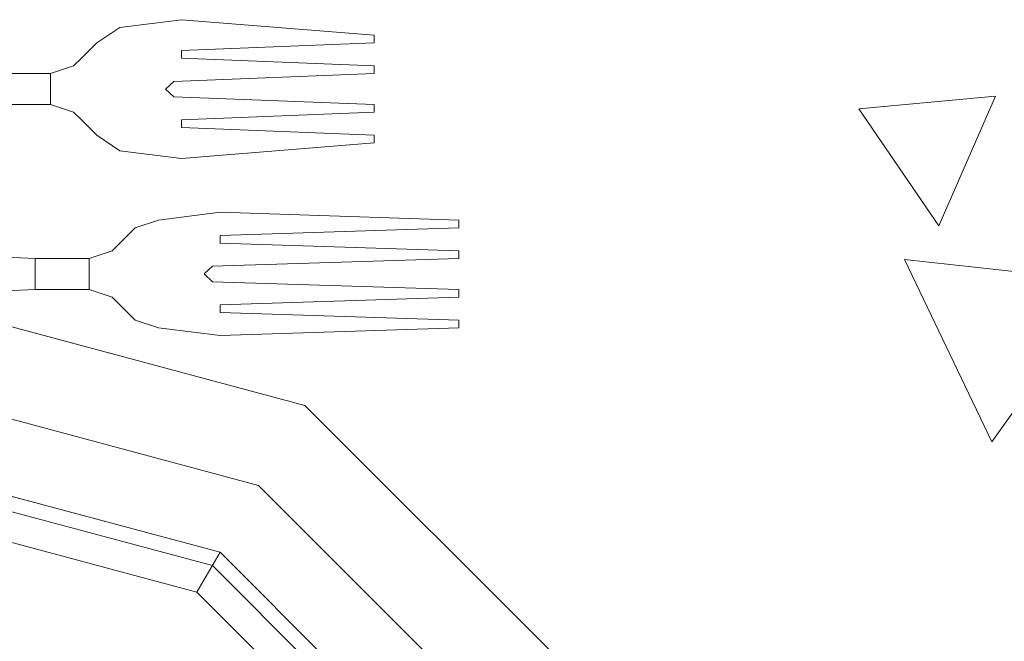
# Model space of a CAD drawing. Units: inches. Extents: x 375 to 1122, y 27 to 1069.
# Tile 25 of 155: x 713 to 721, y 280 to 285. Entities that reach past the tile are written whole.
import ezdxf

# ---------------------------------------------------------------- set-up
doc = ezdxf.new("R2010")
doc.units = ezdxf.units.IN
doc.layers.add('Furniture', color=30, linetype='Continuous', lineweight=18)

# ---------------------------------------------------------------- blocks, each defined once
blk = doc.blocks.new('A$C403C54AD')
for p, q in [((1.57741, 0.87913, -0.0006), (1.58183, 0.91926, -0.0006)), ((1.58183, 0.91926, -0.0006), (1.61385, 0.89659, -0.0006)), ((1.54732, 0.87, -0.0006), (1.54475, 0.89734, -0.0006)), ((1.54475, 0.89734, -0.0006), (1.57064, 0.88596, -0.0006)), ((1.61385, 0.89659, -0.0006), (1.57741, 0.87913, -0.0006)), ((1.57064, 0.88596, -0.0006), (1.54732, 0.87, -0.0006)), ((1.56951, 0.73013, -0.02105), (1.57105, 0.72551, -0.02059)), ((1.56951, 0.73013, -0.02413), (1.57105, 0.72551, -0.02367)), ((1.53103, 0.72244, -0.02105), (1.53411, 0.71782, -0.02059)), ((1.53103, 0.72244, -0.02413), (1.53411, 0.71782, -0.02367))]:
    blk.add_line(p, q)
at = {"linetype": 'ByBlock'}
for points, invisible_edges in [([(1.65725, 0.81008, -0.00874), (1.66648, 0.79408, -0.00874), (1.62254, 0.75014, -0.00874), (1.60654, 0.75938, -0.00874)], 5), ([(1.67418, 0.78075, -0.02259), (1.65725, 0.81008, -0.01335), (1.60654, 0.75938, -0.01335), (1.63587, 0.74244, -0.02259)], 5), ([(1.66648, 0.79408, -0.00874), (1.67572, 0.77809, -0.01489), (1.63853, 0.74091, -0.01489), (1.62254, 0.75014, -0.00874)], 5), ([(1.6788, 0.77276, -0.03183), (1.67418, 0.78075, -0.02259), (1.63587, 0.74244, -0.02259), (1.64387, 0.73783, -0.03183)], 1), ([(1.67572, 0.77809, -0.01489), (1.72651, 0.69011, -0.01489), (1.72651, 0.69011, -0.01489), (1.63853, 0.74091, -0.01489)], 5), ([(1.60654, 0.75938, -0.00874), (1.62254, 0.75014, -0.00874), (1.60645, 0.69011, -0.00874), (1.58798, 0.69011, -0.00874)], 5), ([(1.63587, 0.74244, -0.02259), (1.60654, 0.75938, -0.01335), (1.58798, 0.69011, -0.01335), (1.62185, 0.69011, -0.02259)], 5), ([(1.62254, 0.75014, -0.00874), (1.63853, 0.74091, -0.01489), (1.62492, 0.69011, -0.01489), (1.60645, 0.69011, -0.00874)], 5), ([(1.63853, 0.74091, -0.01489), (1.72651, 0.69011, -0.01489), (1.72651, 0.69011, -0.01489), (1.62492, 0.69011, -0.01489)], 5)]:
    blk.add_3dface(points, dxfattribs=dict(at, invisible_edges=invisible_edges))
for points in [[(1.65725, 0.81008, -0.01335), (1.65725, 0.81008, -0.00874), (1.60654, 0.75938, -0.00874), (1.60654, 0.75938, -0.01335)], [(1.60654, 0.75938, -0.01335), (1.60654, 0.75938, -0.00874), (1.58798, 0.69011, -0.00874), (1.58798, 0.69011, -0.01335)], [(1.64387, 0.73783, -0.03183), (1.63587, 0.74244, -0.02259), (1.62185, 0.69011, -0.02259), (1.63108, 0.69011, -0.03183)]]:
    blk.add_3dface(points, dxfattribs=at)
for points, invisible_edges in [([(1.57259, 0.74244, -0.02045), (1.56797, 0.74244, -0.02045), (1.56951, 0.79016, -0.01335), (1.57105, 0.79016, -0.01335)], 1), ([(1.57259, 0.74244, -0.02353), (1.56797, 0.74244, -0.02353), (1.56951, 0.79016, -0.01643), (1.57105, 0.79016, -0.01643)], 1), ([(1.57875, 0.74091, -0.0207), (1.57413, 0.74244, -0.02045), (1.57567, 0.79016, -0.01335), (1.57721, 0.79016, -0.01335)], 1), ([(1.57875, 0.74091, -0.02378), (1.57413, 0.74244, -0.02353), (1.57567, 0.79016, -0.01643), (1.57721, 0.79016, -0.01643)], 1), ([(1.58645, 0.74244, -0.02045), (1.58183, 0.74091, -0.0207), (1.58337, 0.79016, -0.01335), (1.58491, 0.79016, -0.01335)], 1), ([(1.58645, 0.74244, -0.02353), (1.58183, 0.74091, -0.02378), (1.58337, 0.79016, -0.01643), (1.58491, 0.79016, -0.01643)], 1), ([(1.58798, 0.74244, -0.02045), (1.5926, 0.74244, -0.02045), (1.59106, 0.79016, -0.01335), (1.58952, 0.79016, -0.01335)], 1), ([(1.58798, 0.74244, -0.02353), (1.5926, 0.74244, -0.02353), (1.59106, 0.79016, -0.01643), (1.58952, 0.79016, -0.01643)], 1), ([(1.53565, 0.73475, -0.02045), (1.5295, 0.73475, -0.02045), (1.53257, 0.77323, -0.01335), (1.53411, 0.77323, -0.01335)], 1), ([(1.53565, 0.73475, -0.02353), (1.5295, 0.73475, -0.02353), (1.53257, 0.77323, -0.01643), (1.53411, 0.77323, -0.01643)], 1), ([(1.54181, 0.73321, -0.0207), (1.53719, 0.73475, -0.02045), (1.53873, 0.77323, -0.01335), (1.54027, 0.77323, -0.01335)], 1), ([(1.54181, 0.73321, -0.02378), (1.53719, 0.73475, -0.02353), (1.53873, 0.77323, -0.01643), (1.54027, 0.77323, -0.01643)], 1), ([(1.5495, 0.73475, -0.02045), (1.54489, 0.73321, -0.0207), (1.54643, 0.77323, -0.01335), (1.54797, 0.77323, -0.01335)], 1), ([(1.5495, 0.73475, -0.02353), (1.54489, 0.73321, -0.02378), (1.54643, 0.77323, -0.01643), (1.54797, 0.77323, -0.01643)], 1), ([(1.55104, 0.73475, -0.02045), (1.5572, 0.73475, -0.02045), (1.55412, 0.77323, -0.01335), (1.55258, 0.77323, -0.01335)], 1), ([(1.55104, 0.73475, -0.02353), (1.5572, 0.73475, -0.02353), (1.55412, 0.77323, -0.01643), (1.55258, 0.77323, -0.01643)], 1), ([(1.56951, 0.73013, -0.02105), (1.57413, 0.74244, -0.02045), (1.57259, 0.74244, -0.02045), (1.56797, 0.74244, -0.02045)], 5), ([(1.56951, 0.73013, -0.02413), (1.57413, 0.74244, -0.02353), (1.57259, 0.74244, -0.02353), (1.56797, 0.74244, -0.02353)], 5), ([(1.56951, 0.73013, -0.02413), (1.56951, 0.73013, -0.02105), (1.56797, 0.74244, -0.02045), (1.56797, 0.74244, -0.02353)], 1), ([(1.56951, 0.73013, -0.02105), (1.58029, 0.73924, -0.02085), (1.57875, 0.74091, -0.0207), (1.57413, 0.74244, -0.02045)], 13), ([(1.56951, 0.73013, -0.02413), (1.58029, 0.73924, -0.02392), (1.57875, 0.74091, -0.02378), (1.57413, 0.74244, -0.02353)], 13), ([(1.59106, 0.73013, -0.02105), (1.58029, 0.73924, -0.02085), (1.58183, 0.74091, -0.0207), (1.58645, 0.74244, -0.02045)], 13), ([(1.59106, 0.73013, -0.02413), (1.58029, 0.73924, -0.02392), (1.58183, 0.74091, -0.02378), (1.58645, 0.74244, -0.02353)], 13), ([(1.59106, 0.73013, -0.02105), (1.58645, 0.74244, -0.02045), (1.58798, 0.74244, -0.02045), (1.5926, 0.74244, -0.02045)], 5), ([(1.59106, 0.73013, -0.02413), (1.58645, 0.74244, -0.02353), (1.58798, 0.74244, -0.02353), (1.5926, 0.74244, -0.02353)], 5), ([(1.59106, 0.73013, -0.02105), (1.59106, 0.73013, -0.02413), (1.5926, 0.74244, -0.02353), (1.5926, 0.74244, -0.02045)], 1), ([(1.59106, 0.73013, -0.02105), (1.58029, 0.73924, -0.02085), (1.56951, 0.73013, -0.02105), (1.59106, 0.73013, -0.02105)], 7), ([(1.59106, 0.73013, -0.02413), (1.58029, 0.73924, -0.02392), (1.56951, 0.73013, -0.02413), (1.59106, 0.73013, -0.02413)], 7), ([(1.53103, 0.72244, -0.02105), (1.53719, 0.73475, -0.02045), (1.53565, 0.73475, -0.02045), (1.5295, 0.73475, -0.02045)], 5), ([(1.53103, 0.72244, -0.02413), (1.53719, 0.73475, -0.02353), (1.53565, 0.73475, -0.02353), (1.5295, 0.73475, -0.02353)], 5), ([(1.53103, 0.72244, -0.02413), (1.53103, 0.72244, -0.02105), (1.5295, 0.73475, -0.02045), (1.5295, 0.73475, -0.02353)], 1), ([(1.53103, 0.72244, -0.02105), (1.54335, 0.73155, -0.02085), (1.54181, 0.73321, -0.0207), (1.53719, 0.73475, -0.02045)], 13), ([(1.53103, 0.72244, -0.02413), (1.54335, 0.73155, -0.02392), (1.54181, 0.73321, -0.02378), (1.53719, 0.73475, -0.02353)], 13), ([(1.55566, 0.72244, -0.02105), (1.54335, 0.73155, -0.02085), (1.54489, 0.73321, -0.0207), (1.5495, 0.73475, -0.02045)], 13), ([(1.55566, 0.72244, -0.02413), (1.54335, 0.73155, -0.02392), (1.54489, 0.73321, -0.02378), (1.5495, 0.73475, -0.02353)], 13), ([(1.55566, 0.72244, -0.02105), (1.5495, 0.73475, -0.02045), (1.55104, 0.73475, -0.02045), (1.5572, 0.73475, -0.02045)], 5), ([(1.55566, 0.72244, -0.02413), (1.5495, 0.73475, -0.02353), (1.55104, 0.73475, -0.02353), (1.5572, 0.73475, -0.02353)], 5), ([(1.55566, 0.72244, -0.02105), (1.55566, 0.72244, -0.02413), (1.5572, 0.73475, -0.02353), (1.5572, 0.73475, -0.02045)], 1), ([(1.55566, 0.72244, -0.02105), (1.54335, 0.73155, -0.02085), (1.53103, 0.72244, -0.02105), (1.55566, 0.72244, -0.02105)], 7), ([(1.55566, 0.72244, -0.02413), (1.54335, 0.73155, -0.02392), (1.53103, 0.72244, -0.02413), (1.55566, 0.72244, -0.02413)], 7), ([(1.58952, 0.72551, -0.02059), (1.57105, 0.72551, -0.02059), (1.56951, 0.73013, -0.02105), (1.59106, 0.73013, -0.02105)], 5), ([(1.58952, 0.72551, -0.02367), (1.57105, 0.72551, -0.02367), (1.56951, 0.73013, -0.02413), (1.59106, 0.73013, -0.02413)], 5), ([(1.57105, 0.72551, -0.02059), (1.57105, 0.72551, -0.02367), (1.56951, 0.73013, -0.02413), (1.56951, 0.73013, -0.02105)], 4), ([(1.58952, 0.72551, -0.02367), (1.58952, 0.72551, -0.02059), (1.59106, 0.73013, -0.02105), (1.59106, 0.73013, -0.02413)], 4), ([(1.57413, 0.72244, -0.02243), (1.58645, 0.72244, -0.02243), (1.58952, 0.72551, -0.02367), (1.57105, 0.72551, -0.02367)], 5), ([(1.57413, 0.72244, -0.01935), (1.58645, 0.72244, -0.01935), (1.58952, 0.72551, -0.02059), (1.57105, 0.72551, -0.02059)], 5), ([(1.55258, 0.71782, -0.02059), (1.53411, 0.71782, -0.02059), (1.53103, 0.72244, -0.02105), (1.55566, 0.72244, -0.02105)], 5), ([(1.55258, 0.71782, -0.02367), (1.53411, 0.71782, -0.02367), (1.53103, 0.72244, -0.02413), (1.55566, 0.72244, -0.02413)], 5), ([(1.53411, 0.71782, -0.02059), (1.53411, 0.71782, -0.02367), (1.53103, 0.72244, -0.02413), (1.53103, 0.72244, -0.02105)], 4), ([(1.55258, 0.71782, -0.02367), (1.55258, 0.71782, -0.02059), (1.55566, 0.72244, -0.02105), (1.55566, 0.72244, -0.02413)], 4), ([(1.57567, 0.7209, -0.0183), (1.58491, 0.7209, -0.0183), (1.58645, 0.72244, -0.01935), (1.57413, 0.72244, -0.01935)], 5), ([(1.57567, 0.7209, -0.02109), (1.58491, 0.7209, -0.02109), (1.58645, 0.72244, -0.02243), (1.57413, 0.72244, -0.02243)], 5), ([(1.57567, 0.7209, -0.0183), (1.57567, 0.7209, -0.02109), (1.57413, 0.72244, -0.02243), (1.57413, 0.72244, -0.01935)], 1), ([(1.58491, 0.7209, -0.02109), (1.58491, 0.7209, -0.0183), (1.58645, 0.72244, -0.01935), (1.58645, 0.72244, -0.02243)], 1), ([(1.58337, 0.71628, -0.01595), (1.57721, 0.71628, -0.01595), (1.57567, 0.7209, -0.0183), (1.58491, 0.7209, -0.0183)], 4), ([(1.57721, 0.71628, -0.01854), (1.57721, 0.71628, -0.01595), (1.57567, 0.7209, -0.0183), (1.57567, 0.7209, -0.02109)], 5), ([(1.58337, 0.71628, -0.01854), (1.57721, 0.71628, -0.01854), (1.57567, 0.7209, -0.02109), (1.58491, 0.7209, -0.02109)], 4), ([(1.58337, 0.71628, -0.01595), (1.58337, 0.71628, -0.01854), (1.58491, 0.7209, -0.02109), (1.58491, 0.7209, -0.0183)], 5), ([(1.53719, 0.71474, -0.02243), (1.5495, 0.71474, -0.02243), (1.55258, 0.71782, -0.02367), (1.53411, 0.71782, -0.02367)], 5), ([(1.53719, 0.71474, -0.01935), (1.5495, 0.71474, -0.01935), (1.55258, 0.71782, -0.02059), (1.53411, 0.71782, -0.02059)], 5), ([(1.57721, 0.71628, -0.01854), (1.57721, 0.71628, -0.01595), (1.57721, 0.7055, -0.01387), (1.57721, 0.7055, -0.01646)], 5), ([(1.58337, 0.7055, -0.01646), (1.58337, 0.7055, -0.01387), (1.58337, 0.71628, -0.01595), (1.58337, 0.71628, -0.01854)], 5), ([(1.53873, 0.7132, -0.0183), (1.54797, 0.7132, -0.0183), (1.5495, 0.71474, -0.01935), (1.53719, 0.71474, -0.01935)], 5), ([(1.53873, 0.7132, -0.02109), (1.54797, 0.7132, -0.02109), (1.5495, 0.71474, -0.02243), (1.53719, 0.71474, -0.02243)], 5), ([(1.53873, 0.7132, -0.0183), (1.53873, 0.7132, -0.02109), (1.53719, 0.71474, -0.02243), (1.53719, 0.71474, -0.01935)], 1), ([(1.54797, 0.7132, -0.02109), (1.54797, 0.7132, -0.0183), (1.5495, 0.71474, -0.01935), (1.5495, 0.71474, -0.02243)], 1), ([(1.54643, 0.70858, -0.01595), (1.54027, 0.70858, -0.01595), (1.53873, 0.7132, -0.0183), (1.54797, 0.7132, -0.0183)], 4), ([(1.54643, 0.70858, -0.01854), (1.54027, 0.70858, -0.01854), (1.53873, 0.7132, -0.02109), (1.54797, 0.7132, -0.02109)], 4), ([(1.54027, 0.70858, -0.01854), (1.54027, 0.70858, -0.01595), (1.53873, 0.7132, -0.0183), (1.53873, 0.7132, -0.02109)], 5), ([(1.54643, 0.70858, -0.01595), (1.54643, 0.70858, -0.01854), (1.54797, 0.7132, -0.02109), (1.54797, 0.7132, -0.0183)], 5), ([(1.54027, 0.70858, -0.01854), (1.54027, 0.70858, -0.01595), (1.54027, 0.69781, -0.01387), (1.54027, 0.69781, -0.01646)], 5), ([(1.54643, 0.69781, -0.01646), (1.54643, 0.69781, -0.01387), (1.54643, 0.70858, -0.01595), (1.54643, 0.70858, -0.01854)], 5), ([(1.58491, 0.6701, -0.01678), (1.57567, 0.6701, -0.01678), (1.57721, 0.7055, -0.01387), (1.58337, 0.7055, -0.01387)], 1), ([(1.57721, 0.7055, -0.01387), (1.57721, 0.7055, -0.01646), (1.57567, 0.6701, -0.01986), (1.57567, 0.6701, -0.01678)], 5), ([(1.58491, 0.6701, -0.01986), (1.57567, 0.6701, -0.01986), (1.57721, 0.7055, -0.01646), (1.58337, 0.7055, -0.01646)], 1), ([(1.58491, 0.6701, -0.01678), (1.58491, 0.6701, -0.01986), (1.58337, 0.7055, -0.01646), (1.58337, 0.7055, -0.01387)], 5)]:
    blk.add_3dface(points, dxfattribs=dict(invisible_edges=invisible_edges))
for points in [[(1.56951, 0.79016, -0.01335), (1.56951, 0.79016, -0.01643), (1.56797, 0.74244, -0.02353), (1.56797, 0.74244, -0.02045)], [(1.57105, 0.79016, -0.01643), (1.57105, 0.79016, -0.01335), (1.56951, 0.79016, -0.01335), (1.56951, 0.79016, -0.01643)], [(1.57259, 0.74244, -0.02045), (1.57259, 0.74244, -0.02353), (1.57105, 0.79016, -0.01643), (1.57105, 0.79016, -0.01335)], [(1.57567, 0.79016, -0.01335), (1.57567, 0.79016, -0.01643), (1.57413, 0.74244, -0.02353), (1.57413, 0.74244, -0.02045)], [(1.57721, 0.79016, -0.01643), (1.57721, 0.79016, -0.01335), (1.57567, 0.79016, -0.01335), (1.57567, 0.79016, -0.01643)], [(1.57875, 0.74091, -0.02378), (1.57875, 0.74091, -0.0207), (1.57721, 0.79016, -0.01335), (1.57721, 0.79016, -0.01643)], [(1.58337, 0.79016, -0.01643), (1.58337, 0.79016, -0.01335), (1.58183, 0.74091, -0.0207), (1.58183, 0.74091, -0.02378)], [(1.58491, 0.79016, -0.01643), (1.58491, 0.79016, -0.01335), (1.58337, 0.79016, -0.01335), (1.58337, 0.79016, -0.01643)], [(1.58645, 0.74244, -0.02353), (1.58645, 0.74244, -0.02045), (1.58491, 0.79016, -0.01335), (1.58491, 0.79016, -0.01643)], [(1.58952, 0.79016, -0.01335), (1.58952, 0.79016, -0.01643), (1.58798, 0.74244, -0.02353), (1.58798, 0.74244, -0.02045)], [(1.59106, 0.79016, -0.01643), (1.59106, 0.79016, -0.01335), (1.58952, 0.79016, -0.01335), (1.58952, 0.79016, -0.01643)], [(1.5926, 0.74244, -0.02353), (1.5926, 0.74244, -0.02045), (1.59106, 0.79016, -0.01335), (1.59106, 0.79016, -0.01643)], [(1.53257, 0.77323, -0.01335), (1.53257, 0.77323, -0.01643), (1.5295, 0.73475, -0.02353), (1.5295, 0.73475, -0.02045)], [(1.53411, 0.77323, -0.01643), (1.53411, 0.77323, -0.01335), (1.53257, 0.77323, -0.01335), (1.53257, 0.77323, -0.01643)], [(1.53565, 0.73475, -0.02045), (1.53565, 0.73475, -0.02353), (1.53411, 0.77323, -0.01643), (1.53411, 0.77323, -0.01335)], [(1.53873, 0.77323, -0.01335), (1.53873, 0.77323, -0.01643), (1.53719, 0.73475, -0.02353), (1.53719, 0.73475, -0.02045)], [(1.54027, 0.77323, -0.01643), (1.54027, 0.77323, -0.01335), (1.53873, 0.77323, -0.01335), (1.53873, 0.77323, -0.01643)], [(1.54181, 0.73321, -0.02378), (1.54181, 0.73321, -0.0207), (1.54027, 0.77323, -0.01335), (1.54027, 0.77323, -0.01643)], [(1.54643, 0.77323, -0.01643), (1.54643, 0.77323, -0.01335), (1.54489, 0.73321, -0.0207), (1.54489, 0.73321, -0.02378)], [(1.54797, 0.77323, -0.01643), (1.54797, 0.77323, -0.01335), (1.54643, 0.77323, -0.01335), (1.54643, 0.77323, -0.01643)], [(1.5495, 0.73475, -0.02353), (1.5495, 0.73475, -0.02045), (1.54797, 0.77323, -0.01335), (1.54797, 0.77323, -0.01643)], [(1.55258, 0.77323, -0.01335), (1.55258, 0.77323, -0.01643), (1.55104, 0.73475, -0.02353), (1.55104, 0.73475, -0.02045)], [(1.55412, 0.77323, -0.01643), (1.55412, 0.77323, -0.01335), (1.55258, 0.77323, -0.01335), (1.55258, 0.77323, -0.01643)], [(1.5572, 0.73475, -0.02353), (1.5572, 0.73475, -0.02045), (1.55412, 0.77323, -0.01335), (1.55412, 0.77323, -0.01643)], [(1.57259, 0.74244, -0.02045), (1.57259, 0.74244, -0.02353), (1.57413, 0.74244, -0.02353), (1.57413, 0.74244, -0.02045)], [(1.58645, 0.74244, -0.02353), (1.58645, 0.74244, -0.02045), (1.58798, 0.74244, -0.02045), (1.58798, 0.74244, -0.02353)], [(1.57875, 0.74091, -0.0207), (1.57875, 0.74091, -0.02378), (1.58029, 0.73924, -0.02392), (1.58029, 0.73924, -0.02085)], [(1.58029, 0.73924, -0.02392), (1.58029, 0.73924, -0.02085), (1.58183, 0.74091, -0.0207), (1.58183, 0.74091, -0.02378)], [(1.53565, 0.73475, -0.02045), (1.53565, 0.73475, -0.02353), (1.53719, 0.73475, -0.02353), (1.53719, 0.73475, -0.02045)], [(1.5495, 0.73475, -0.02353), (1.5495, 0.73475, -0.02045), (1.55104, 0.73475, -0.02045), (1.55104, 0.73475, -0.02353)], [(1.54181, 0.73321, -0.0207), (1.54181, 0.73321, -0.02378), (1.54335, 0.73155, -0.02392), (1.54335, 0.73155, -0.02085)], [(1.54335, 0.73155, -0.02392), (1.54335, 0.73155, -0.02085), (1.54489, 0.73321, -0.0207), (1.54489, 0.73321, -0.02378)], [(1.57413, 0.72244, -0.02243), (1.57413, 0.72244, -0.01935), (1.57105, 0.72551, -0.02059), (1.57105, 0.72551, -0.02367)], [(1.58645, 0.72244, -0.01935), (1.58645, 0.72244, -0.02243), (1.58952, 0.72551, -0.02367), (1.58952, 0.72551, -0.02059)], [(1.53719, 0.71474, -0.02243), (1.53719, 0.71474, -0.01935), (1.53411, 0.71782, -0.02059), (1.53411, 0.71782, -0.02367)], [(1.5495, 0.71474, -0.01935), (1.5495, 0.71474, -0.02243), (1.55258, 0.71782, -0.02367), (1.55258, 0.71782, -0.02059)], [(1.57721, 0.7055, -0.01387), (1.58337, 0.7055, -0.01387), (1.58337, 0.71628, -0.01595), (1.57721, 0.71628, -0.01595)], [(1.57721, 0.7055, -0.01646), (1.58337, 0.7055, -0.01646), (1.58337, 0.71628, -0.01854), (1.57721, 0.71628, -0.01854)], [(1.54027, 0.69781, -0.01387), (1.54643, 0.69781, -0.01387), (1.54643, 0.70858, -0.01595), (1.54027, 0.70858, -0.01595)], [(1.54027, 0.69781, -0.01646), (1.54643, 0.69781, -0.01646), (1.54643, 0.70858, -0.01854), (1.54027, 0.70858, -0.01854)]]:
    blk.add_3dface(points)

msp = doc.modelspace()

# ---------------------------------------------------------------- block references
at = {"layer": 'Furniture', "xscale": 39.9918517141215, "yscale": 39.9918517141215, "zscale": 39.9918517141215, "rotation": 270}
msp.add_blockref('A$C403C54AD', (684.9549, 346.2875, 0.024), dxfattribs=at)

doc.saveas('drawing.dxf')
